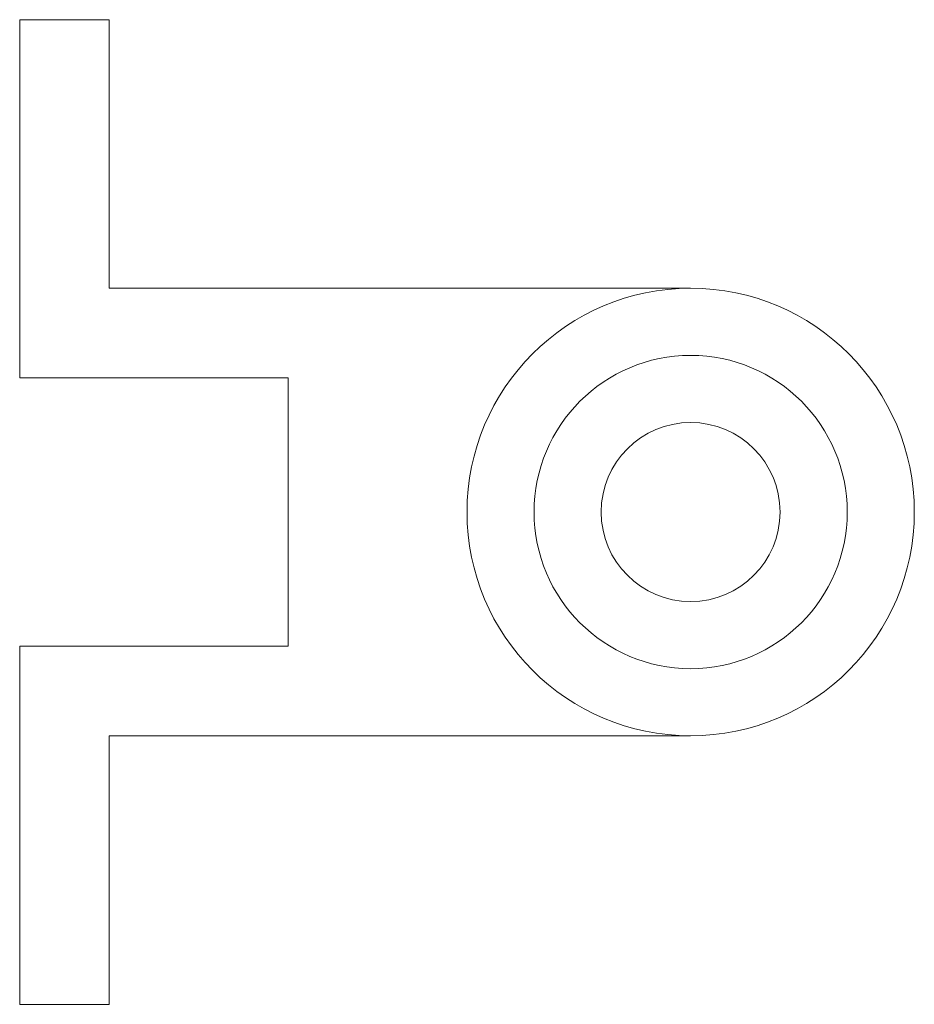
# Model space of a CAD drawing. Units: millimetres. Extents: x 1854 to 1954, y -339 to -229.
import ezdxf

# ---------------------------------------------------------------- set-up
doc = ezdxf.new("R2010")
doc.units = ezdxf.units.MM
doc.layers.add('M-CONS', color=8, linetype='Continuous', lineweight=18)

msp = doc.modelspace()

# ---------------------------------------------------------------- linework, layer by layer
at = {"layer": 'M-CONS'}
for p, q in [((1853.92, -269.36), (1853.92, -229.36)), ((1863.92, -229.36), (1853.92, -229.36)), ((1863.92, -229.36), (1863.92, -259.36)), ((1863.92, -259.36), (1928.92, -259.36)), ((1883.92, -269.36), (1853.92, -269.36)), ((1883.92, -299.36), (1883.92, -269.36)), ((1853.92, -329.36), (1853.92, -299.36)), ((1853.92, -299.36), (1883.92, -299.36)), ((1928.92, -309.36), (1863.92, -309.36)), ((1863.92, -309.36), (1863.92, -339.36)), ((1853.92, -339.36), (1853.92, -329.36)), ((1863.92, -339.36), (1853.92, -339.36))]:
    msp.add_line(p, q, dxfattribs=at)
at = {"layer": 'M-CONS', "extrusion": (0, -1, 0)}
msp.add_line((1863.92, -339.36), (1863.92, -339.36), dxfattribs=at)
msp.add_line((1863.92, -339.36), (1863.92, -339.36), dxfattribs=at)
at = {"layer": 'M-CONS'}
for radius in [25, 17.5, 10]:
    msp.add_circle((1928.92, -284.36), radius, dxfattribs=at)
msp.add_arc((1928.92, -284.36), 25, 90, 270, dxfattribs=at)

doc.saveas('drawing.dxf')
